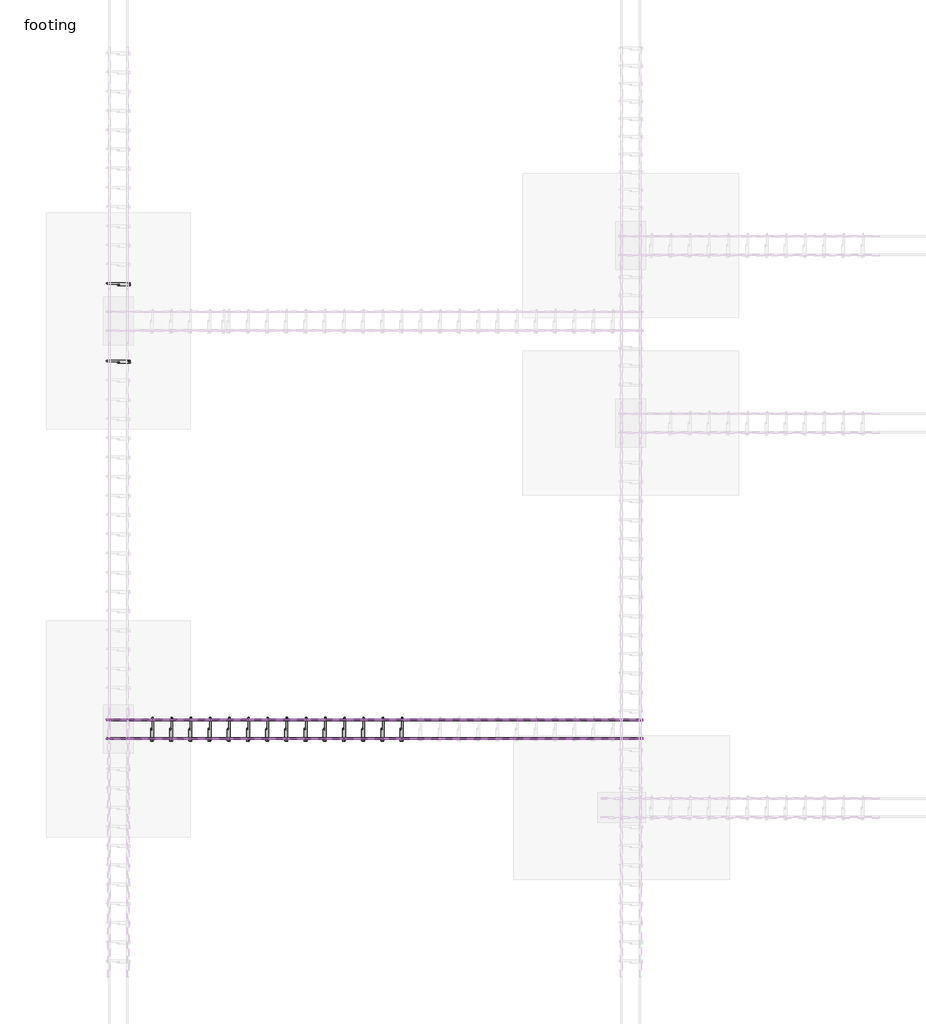
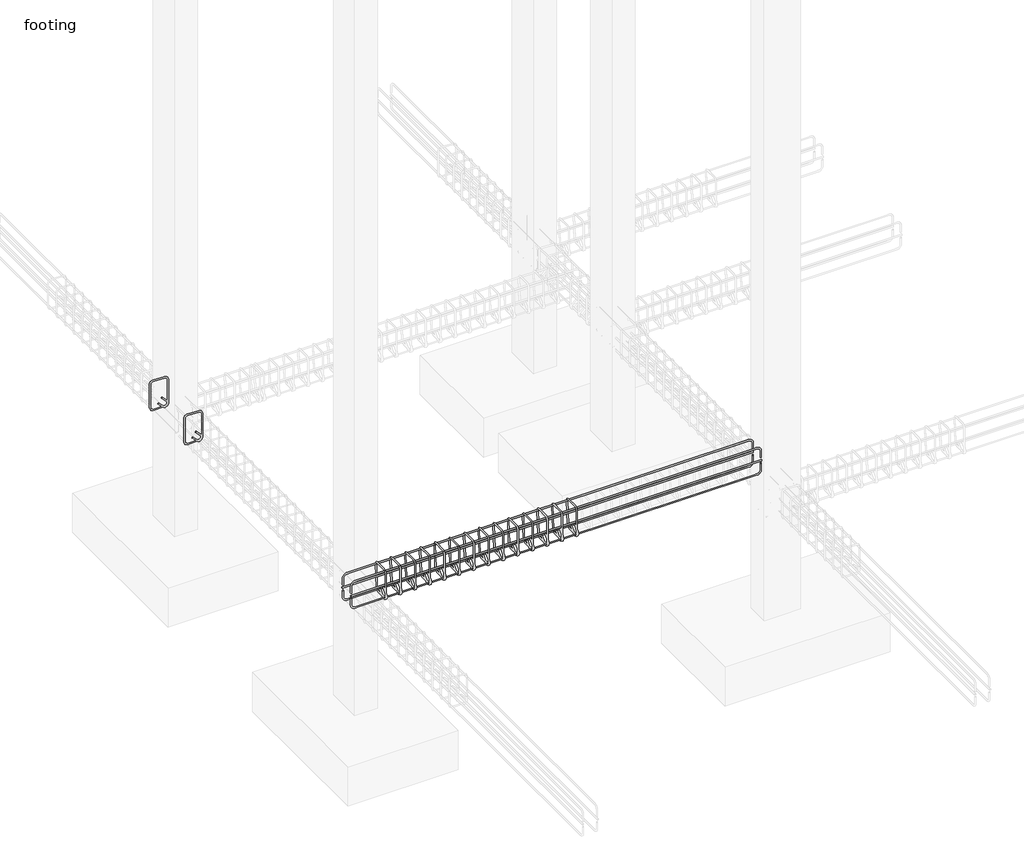
# One storey, part 6 of 21: 22 reinforcing bars.
"""IFC4 building model written with IfcOpenShell, lengths in millimetres."""

from ifc_helpers import new_model, si_unit, point, frame, origin, place, context, project, spatial, polyline, circle_curve, trimmed, segment, composite_curve, element, save
from ifc_brep_helpers import swept_disk

model = new_model("IFC4")

# Units and contexts
model_context = context("Model", 3, world=origin())
ifc_project = project(units=[si_unit("LENGTHUNIT", "METRE", prefix="MILLI")], contexts=[model_context])

# Site, building, storey
site = spatial("IfcSite", under=ifc_project)
building = spatial("IfcBuilding", under=site)
storey = spatial("IfcBuildingStorey", under=building, Name="footing", Elevation=-1524.0)

# Reinforcing bars
placement = place(None, origin())
element("IfcReinforcingBar", 1, at=placement, inside=storey, context=model_context, shape_type="SolidModel", body=[
    swept_disk(composite_curve([segment(polyline([(-10142.5883428, 4117.8887132, -310.8825168), (-10142.5883428, 4063.0237147, -365.7475153)]), True, "CONTINUOUS"), segment(trimmed(circle_curve(frame((-10142.5883428, 4040.5730744, -343.296875), z_axis=(-1.0, 0.0, 0.0), x_axis=(0.0, 22.450640299999577, -22.450640299999975)), 31.75), [point((-10142.5883428, 4063.0237147, -365.7475153))], [point((-10142.5883428, 4008.8230744, -343.296875))], True, "CARTESIAN"), True, "CONTINUOUS"), segment(polyline([(-10142.5883428, 4008.8230744, -343.296875), (-10142.5883428, 4008.8230744, -63.103125)]), True, "CONTINUOUS"), segment(trimmed(circle_curve(frame((-10142.5883428, 4040.5730744, -63.103125), z_axis=(-1.0, 0.0, 0.0), x_axis=(0.0, -31.75, 0.0)), 31.75), [point((-10142.5883428, 4008.8230744, -63.103125))], [point((-10142.5883428, 4040.5730744, -31.353125))], True, "CARTESIAN"), True, "CONTINUOUS"), segment(polyline([(-10142.5883428, 4040.5730744, -31.353125), (-10142.5883428, 4168.3668244, -31.353125)]), True, "CONTINUOUS"), segment(trimmed(circle_curve(frame((-10141.4159328, 4168.3668244, -63.0814712), z_axis=(-0.9993179916193466, 0.0, -0.03692629992126919), x_axis=(-1.1724099999992177, 0.0, 31.728346200000004)), 31.75), [point((-10142.5883428, 4168.3668244, -31.353125))], [point((-10141.4159328, 4200.1168244, -63.0814712))], True, "CARTESIAN"), True, "CONTINUOUS"), segment(polyline([(-10141.4159328, 4200.1168244, -63.0814712), (-10131.0607528, 4200.1168244, -343.3185288)]), True, "CONTINUOUS"), segment(trimmed(circle_curve(frame((-10131.0607528, 4168.3668244, -343.3185288), z_axis=(-0.9993179916193466, 0.0, -0.03692629992126919), x_axis=(0.0, 31.75, 0.0)), 31.75), [point((-10131.0607528, 4200.1168244, -343.3185288))], [point((-10129.8883428, 4168.3668244, -375.046875))], True, "CARTESIAN"), True, "CONTINUOUS"), segment(polyline([(-10129.8883428, 4168.3668244, -375.046875), (-10129.8883428, 4040.5730744, -375.046875)]), True, "CONTINUOUS"), segment(trimmed(circle_curve(frame((-10129.8883428, 4040.5730744, -343.296875), z_axis=(-1.0, 0.0, 0.0), x_axis=(0.0, 0.0, -31.75)), 31.75), [point((-10129.8883428, 4040.5730744, -375.046875))], [point((-10129.8883428, 4018.1224341, -320.8462347))], True, "CARTESIAN"), True, "CONTINUOUS"), segment(polyline([(-10129.8883428, 4018.1224341, -320.8462347), (-10129.8883428, 4072.9874326, -265.9812362)]), True, "CONTINUOUS")], self_intersect=False), 6.35),
])
element("IfcReinforcingBar", 2, at=placement, inside=storey, context=model_context, shape_type="SolidModel", body=[
    swept_disk(composite_curve([segment(polyline([(-9979.8883428, 4117.8887132, -310.8825168), (-9979.8883428, 4063.0237147, -365.7475153)]), True, "CONTINUOUS"), segment(trimmed(circle_curve(frame((-9979.8883428, 4040.5730744, -343.296875), z_axis=(-1.0, 0.0, 0.0), x_axis=(0.0, 22.450640299999577, -22.450640299999975)), 31.75), [point((-9979.8883428, 4063.0237147, -365.7475153))], [point((-9979.8883428, 4008.8230744, -343.296875))], True, "CARTESIAN"), True, "CONTINUOUS"), segment(polyline([(-9979.8883428, 4008.8230744, -343.296875), (-9979.8883428, 4008.8230744, -63.103125)]), True, "CONTINUOUS"), segment(trimmed(circle_curve(frame((-9979.8883428, 4040.5730744, -63.103125), z_axis=(-1.0, 0.0, 0.0), x_axis=(0.0, -31.75, 0.0)), 31.75), [point((-9979.8883428, 4008.8230744, -63.103125))], [point((-9979.8883428, 4040.5730744, -31.353125))], True, "CARTESIAN"), True, "CONTINUOUS"), segment(polyline([(-9979.8883428, 4040.5730744, -31.353125), (-9979.8883428, 4168.3668244, -31.353125)]), True, "CONTINUOUS"), segment(trimmed(circle_curve(frame((-9978.7159328, 4168.3668244, -63.0814712), z_axis=(-0.9993179916193466, 0.0, -0.03692629992126919), x_axis=(-1.1724100000010367, 0.0, 31.728346200000004)), 31.75), [point((-9979.8883428, 4168.3668244, -31.353125))], [point((-9978.7159328, 4200.1168244, -63.0814712))], True, "CARTESIAN"), True, "CONTINUOUS"), segment(polyline([(-9978.7159328, 4200.1168244, -63.0814712), (-9968.3607528, 4200.1168244, -343.3185288)]), True, "CONTINUOUS"), segment(trimmed(circle_curve(frame((-9968.3607528, 4168.3668244, -343.3185288), z_axis=(-0.9993179916193466, 0.0, -0.03692629992126919), x_axis=(0.0, 31.75, 0.0)), 31.75), [point((-9968.3607528, 4200.1168244, -343.3185288))], [point((-9967.1883428, 4168.3668244, -375.046875))], True, "CARTESIAN"), True, "CONTINUOUS"), segment(polyline([(-9967.1883428, 4168.3668244, -375.046875), (-9967.1883428, 4040.5730744, -375.046875)]), True, "CONTINUOUS"), segment(trimmed(circle_curve(frame((-9967.1883428, 4040.5730744, -343.296875), z_axis=(-1.0, 0.0, 0.0), x_axis=(0.0, 0.0, -31.75)), 31.75), [point((-9967.1883428, 4040.5730744, -375.046875))], [point((-9967.1883428, 4018.1224341, -320.8462347))], True, "CARTESIAN"), True, "CONTINUOUS"), segment(polyline([(-9967.1883428, 4018.1224341, -320.8462347), (-9967.1883428, 4072.9874326, -265.9812362)]), True, "CONTINUOUS")], self_intersect=False), 6.35),
])
element("IfcReinforcingBar", 3, at=placement, inside=storey, context=model_context, shape_type="SolidModel", body=[
    swept_disk(composite_curve([segment(polyline([(-9817.1883428, 4117.8887132, -310.8825168), (-9817.1883428, 4063.0237147, -365.7475153)]), True, "CONTINUOUS"), segment(trimmed(circle_curve(frame((-9817.1883428, 4040.5730744, -343.296875), z_axis=(-1.0, 0.0, 0.0), x_axis=(0.0, 22.450640299999577, -22.450640299999975)), 31.75), [point((-9817.1883428, 4063.0237147, -365.7475153))], [point((-9817.1883428, 4008.8230744, -343.296875))], True, "CARTESIAN"), True, "CONTINUOUS"), segment(polyline([(-9817.1883428, 4008.8230744, -343.296875), (-9817.1883428, 4008.8230744, -63.103125)]), True, "CONTINUOUS"), segment(trimmed(circle_curve(frame((-9817.1883428, 4040.5730744, -63.103125), z_axis=(-1.0, 0.0, 0.0), x_axis=(0.0, -31.75, 0.0)), 31.75), [point((-9817.1883428, 4008.8230744, -63.103125))], [point((-9817.1883428, 4040.5730744, -31.353125))], True, "CARTESIAN"), True, "CONTINUOUS"), segment(polyline([(-9817.1883428, 4040.5730744, -31.353125), (-9817.1883428, 4168.3668244, -31.353125)]), True, "CONTINUOUS"), segment(trimmed(circle_curve(frame((-9816.0159328, 4168.3668244, -63.0814712), z_axis=(-0.9993179916193466, 0.0, -0.03692629992126919), x_axis=(-1.1724099999992177, 0.0, 31.728346200000004)), 31.75), [point((-9817.1883428, 4168.3668244, -31.353125))], [point((-9816.0159328, 4200.1168244, -63.0814712))], True, "CARTESIAN"), True, "CONTINUOUS"), segment(polyline([(-9816.0159328, 4200.1168244, -63.0814712), (-9805.6607528, 4200.1168244, -343.3185288)]), True, "CONTINUOUS"), segment(trimmed(circle_curve(frame((-9805.6607528, 4168.3668244, -343.3185288), z_axis=(-0.9993179916193466, 0.0, -0.03692629992126919), x_axis=(0.0, 31.75, 0.0)), 31.75), [point((-9805.6607528, 4200.1168244, -343.3185288))], [point((-9804.4883428, 4168.3668244, -375.046875))], True, "CARTESIAN"), True, "CONTINUOUS"), segment(polyline([(-9804.4883428, 4168.3668244, -375.046875), (-9804.4883428, 4040.5730744, -375.046875)]), True, "CONTINUOUS"), segment(trimmed(circle_curve(frame((-9804.4883428, 4040.5730744, -343.296875), z_axis=(-1.0, 0.0, 0.0), x_axis=(0.0, 0.0, -31.75)), 31.75), [point((-9804.4883428, 4040.5730744, -375.046875))], [point((-9804.4883428, 4018.1224341, -320.8462347))], True, "CARTESIAN"), True, "CONTINUOUS"), segment(polyline([(-9804.4883428, 4018.1224341, -320.8462347), (-9804.4883428, 4072.9874326, -265.9812362)]), True, "CONTINUOUS")], self_intersect=False), 6.35),
])
element("IfcReinforcingBar", 4, at=placement, inside=storey, context=model_context, shape_type="SolidModel", body=[
    swept_disk(composite_curve([segment(polyline([(-7770.5521673, 4181.8372086, -236.1172592), (-7770.5521673, 4181.8372086, -312.3172592)]), True, "CONTINUOUS"), segment(trimmed(circle_curve(frame((-7815.0021673, 4181.8372086, -312.3172592), z_axis=(0.0, 1.0, -2.1166279873208456e-12), x_axis=(44.44999999999982, 0.0, 0.0)), 44.45), [point((-7770.5521673, 4181.8372086, -312.3172592))], [point((-7815.0021673, 4181.8372086, -356.7672592))], True, "CARTESIAN"), True, "CONTINUOUS"), segment(polyline([(-7815.0021673, 4181.8372086, -356.7672592), (-12260.7959173, 4181.8372086, -356.7672592)]), True, "CONTINUOUS"), segment(trimmed(circle_curve(frame((-12260.7959173, 4181.8372086, -312.3172592), z_axis=(0.0, 1.0, -2.1166279873208456e-12), x_axis=(0.0, 0.0, -44.44999999999999)), 44.45), [point((-12260.7959173, 4181.8372086, -356.7672592))], [point((-12305.2459173, 4181.8372086, -312.3172592))], True, "CARTESIAN"), True, "CONTINUOUS"), segment(polyline([(-12305.2459173, 4181.8372086, -312.3172592), (-12305.2459173, 4181.8372086, -236.1172592)]), True, "CONTINUOUS")], self_intersect=False), 6.35),
])
element("IfcReinforcingBar", 5, at=placement, inside=storey, context=model_context, shape_type="SolidModel", body=[
    swept_disk(composite_curve([segment(polyline([(-7770.5521673, 4027.1026902, -170.2827408), (-7770.5521673, 4027.1026902, -94.0827408)]), True, "CONTINUOUS"), segment(trimmed(circle_curve(frame((-7815.0021673, 4027.1026902, -94.0827408), z_axis=(0.0, -1.0, 0.0), x_axis=(44.44999999999982, 0.0, 0.0)), 44.45), [point((-7770.5521673, 4027.1026902, -94.0827408))], [point((-7815.0021673, 4027.1026902, -49.6327408))], True, "CARTESIAN"), True, "CONTINUOUS"), segment(polyline([(-7815.0021673, 4027.1026902, -49.6327408), (-12260.7959173, 4027.1026902, -49.6327408)]), True, "CONTINUOUS"), segment(trimmed(circle_curve(frame((-12260.7959173, 4027.1026902, -94.0827408), z_axis=(0.0, -1.0, 0.0), x_axis=(0.0, 0.0, 44.449999999999996)), 44.45), [point((-12260.7959173, 4027.1026902, -49.6327408))], [point((-12305.2459173, 4027.1026902, -94.0827408))], True, "CARTESIAN"), True, "CONTINUOUS"), segment(polyline([(-12305.2459173, 4027.1026902, -94.0827408), (-12305.2459173, 4027.1026902, -170.2827408)]), True, "CONTINUOUS")], self_intersect=False), 6.35),
])
element("IfcReinforcingBar", 6, at=placement, inside=storey, context=model_context, shape_type="SolidModel", body=[
    swept_disk(composite_curve([segment(polyline([(-7770.5521673, 4027.1026902, -236.1172592), (-7770.5521673, 4027.1026902, -312.3172592)]), True, "CONTINUOUS"), segment(trimmed(circle_curve(frame((-7815.0021673, 4027.1026902, -312.3172592), z_axis=(0.0, 1.0, 2.1166279873208456e-12), x_axis=(44.44999999999982, 0.0, 0.0)), 44.45), [point((-7770.5521673, 4027.1026902, -312.3172592))], [point((-7815.0021673, 4027.1026902, -356.7672592))], True, "CARTESIAN"), True, "CONTINUOUS"), segment(polyline([(-7815.0021673, 4027.1026902, -356.7672592), (-12260.7959173, 4027.1026902, -356.7672592)]), True, "CONTINUOUS"), segment(trimmed(circle_curve(frame((-12260.7959173, 4027.1026902, -312.3172592), z_axis=(0.0, 1.0, 2.1166279873208456e-12), x_axis=(0.0, 0.0, -44.44999999999999)), 44.45), [point((-12260.7959173, 4027.1026902, -356.7672592))], [point((-12305.2459173, 4027.1026902, -312.3172592))], True, "CARTESIAN"), True, "CONTINUOUS"), segment(polyline([(-12305.2459173, 4027.1026902, -312.3172592), (-12305.2459173, 4027.1026902, -236.1172592)]), True, "CONTINUOUS")], self_intersect=False), 6.35),
])
element("IfcReinforcingBar", 7, at=placement, inside=storey, context=model_context, shape_type="SolidModel", body=[
    swept_disk(composite_curve([segment(polyline([(-7770.5521673, 4181.8372086, -170.2827408), (-7770.5521673, 4181.8372086, -94.0827408)]), True, "CONTINUOUS"), segment(trimmed(circle_curve(frame((-7815.0021673, 4181.8372086, -94.0827408), z_axis=(0.0, -1.0, 0.0), x_axis=(44.44999999999982, 0.0, 0.0)), 44.45), [point((-7770.5521673, 4181.8372086, -94.0827408))], [point((-7815.0021673, 4181.8372086, -49.6327408))], True, "CARTESIAN"), True, "CONTINUOUS"), segment(polyline([(-7815.0021673, 4181.8372086, -49.6327408), (-12260.7959173, 4181.8372086, -49.6327408)]), True, "CONTINUOUS"), segment(trimmed(circle_curve(frame((-12260.7959173, 4181.8372086, -94.0827408), z_axis=(0.0, -1.0, 0.0), x_axis=(0.0, 0.0, 44.449999999999996)), 44.45), [point((-12260.7959173, 4181.8372086, -49.6327408))], [point((-12305.2459173, 4181.8372086, -94.0827408))], True, "CARTESIAN"), True, "CONTINUOUS"), segment(polyline([(-12305.2459173, 4181.8372086, -94.0827408), (-12305.2459173, 4181.8372086, -170.2827408)]), True, "CONTINUOUS")], self_intersect=False), 6.35),
])
element("IfcReinforcingBar", 8, at=placement, inside=storey, context=model_context, shape_type="SolidModel", body=[
    swept_disk(composite_curve([segment(polyline([(-7764.2021673, 4187.4168244, -203.2), (-12311.5959173, 4187.4168244, -203.2)]), True, "CONTINUOUS")], self_intersect=False), 6.35),
])
element("IfcReinforcingBar", 9, at=placement, inside=storey, context=model_context, shape_type="SolidModel", body=[
    swept_disk(composite_curve([segment(polyline([(-7764.2021673, 4021.5230744, -203.2), (-12311.5959173, 4021.5230744, -203.2)]), True, "CONTINUOUS")], self_intersect=False), 6.35),
])
element("IfcReinforcingBar", 10, at=placement, inside=storey, context=model_context, shape_type="SolidModel", body=[
    swept_disk(composite_curve([segment(polyline([(-10305.2883428, 4117.8887132, -310.8825168), (-10305.2883428, 4063.0237147, -365.7475153)]), True, "CONTINUOUS"), segment(trimmed(circle_curve(frame((-10305.2883428, 4040.5730744, -343.296875), z_axis=(-1.0, 0.0, 0.0), x_axis=(0.0, 22.450640299999577, -22.450640299999975)), 31.75), [point((-10305.2883428, 4063.0237147, -365.7475153))], [point((-10305.2883428, 4008.8230744, -343.296875))], True, "CARTESIAN"), True, "CONTINUOUS"), segment(polyline([(-10305.2883428, 4008.8230744, -343.296875), (-10305.2883428, 4008.8230744, -63.103125)]), True, "CONTINUOUS"), segment(trimmed(circle_curve(frame((-10305.2883428, 4040.5730744, -63.103125), z_axis=(-1.0, 0.0, 0.0), x_axis=(0.0, -31.75, 0.0)), 31.75), [point((-10305.2883428, 4008.8230744, -63.103125))], [point((-10305.2883428, 4040.5730744, -31.353125))], True, "CARTESIAN"), True, "CONTINUOUS"), segment(polyline([(-10305.2883428, 4040.5730744, -31.353125), (-10305.2883428, 4168.3668244, -31.353125)]), True, "CONTINUOUS"), segment(trimmed(circle_curve(frame((-10304.1159328, 4168.3668244, -63.0814712), z_axis=(-0.9993179916193466, 0.0, -0.03692629992126919), x_axis=(-1.1724100000010367, 0.0, 31.728346200000004)), 31.75), [point((-10305.2883428, 4168.3668244, -31.353125))], [point((-10304.1159328, 4200.1168244, -63.0814712))], True, "CARTESIAN"), True, "CONTINUOUS"), segment(polyline([(-10304.1159328, 4200.1168244, -63.0814712), (-10293.7607528, 4200.1168244, -343.3185288)]), True, "CONTINUOUS"), segment(trimmed(circle_curve(frame((-10293.7607528, 4168.3668244, -343.3185288), z_axis=(-0.9993179916193466, 0.0, -0.03692629992126919), x_axis=(0.0, 31.75, 0.0)), 31.75), [point((-10293.7607528, 4200.1168244, -343.3185288))], [point((-10292.5883428, 4168.3668244, -375.046875))], True, "CARTESIAN"), True, "CONTINUOUS"), segment(polyline([(-10292.5883428, 4168.3668244, -375.046875), (-10292.5883428, 4040.5730744, -375.046875)]), True, "CONTINUOUS"), segment(trimmed(circle_curve(frame((-10292.5883428, 4040.5730744, -343.296875), z_axis=(-1.0, 0.0, 0.0), x_axis=(0.0, 0.0, -31.75)), 31.75), [point((-10292.5883428, 4040.5730744, -375.046875))], [point((-10292.5883428, 4018.1224341, -320.8462347))], True, "CARTESIAN"), True, "CONTINUOUS"), segment(polyline([(-10292.5883428, 4018.1224341, -320.8462347), (-10292.5883428, 4072.9874326, -265.9812362)]), True, "CONTINUOUS")], self_intersect=False), 6.35),
])
element("IfcReinforcingBar", 11, at=placement, inside=storey, context=model_context, shape_type="SolidModel", body=[
    swept_disk(composite_curve([segment(polyline([(-10467.9883428, 4117.8887132, -310.8825168), (-10467.9883428, 4063.0237147, -365.7475153)]), True, "CONTINUOUS"), segment(trimmed(circle_curve(frame((-10467.9883428, 4040.5730744, -343.296875), z_axis=(-1.0, 0.0, 0.0), x_axis=(0.0, 22.450640299999577, -22.450640299999975)), 31.75), [point((-10467.9883428, 4063.0237147, -365.7475153))], [point((-10467.9883428, 4008.8230744, -343.296875))], True, "CARTESIAN"), True, "CONTINUOUS"), segment(polyline([(-10467.9883428, 4008.8230744, -343.296875), (-10467.9883428, 4008.8230744, -63.103125)]), True, "CONTINUOUS"), segment(trimmed(circle_curve(frame((-10467.9883428, 4040.5730744, -63.103125), z_axis=(-1.0, 0.0, 0.0), x_axis=(0.0, -31.75, 0.0)), 31.75), [point((-10467.9883428, 4008.8230744, -63.103125))], [point((-10467.9883428, 4040.5730744, -31.353125))], True, "CARTESIAN"), True, "CONTINUOUS"), segment(polyline([(-10467.9883428, 4040.5730744, -31.353125), (-10467.9883428, 4168.3668244, -31.353125)]), True, "CONTINUOUS"), segment(trimmed(circle_curve(frame((-10466.8159328, 4168.3668244, -63.0814712), z_axis=(-0.9993179916193466, 0.0, -0.03692629992126919), x_axis=(-1.1724099999992177, 0.0, 31.728346200000004)), 31.75), [point((-10467.9883428, 4168.3668244, -31.353125))], [point((-10466.8159328, 4200.1168244, -63.0814712))], True, "CARTESIAN"), True, "CONTINUOUS"), segment(polyline([(-10466.8159328, 4200.1168244, -63.0814712), (-10456.4607528, 4200.1168244, -343.3185288)]), True, "CONTINUOUS"), segment(trimmed(circle_curve(frame((-10456.4607528, 4168.3668244, -343.3185288), z_axis=(-0.9993179916193466, 0.0, -0.03692629992126919), x_axis=(0.0, 31.75, 0.0)), 31.75), [point((-10456.4607528, 4200.1168244, -343.3185288))], [point((-10455.2883428, 4168.3668244, -375.046875))], True, "CARTESIAN"), True, "CONTINUOUS"), segment(polyline([(-10455.2883428, 4168.3668244, -375.046875), (-10455.2883428, 4040.5730744, -375.046875)]), True, "CONTINUOUS"), segment(trimmed(circle_curve(frame((-10455.2883428, 4040.5730744, -343.296875), z_axis=(-1.0, 0.0, 0.0), x_axis=(0.0, 0.0, -31.75)), 31.75), [point((-10455.2883428, 4040.5730744, -375.046875))], [point((-10455.2883428, 4018.1224341, -320.8462347))], True, "CARTESIAN"), True, "CONTINUOUS"), segment(polyline([(-10455.2883428, 4018.1224341, -320.8462347), (-10455.2883428, 4072.9874326, -265.9812362)]), True, "CONTINUOUS")], self_intersect=False), 6.35),
])
element("IfcReinforcingBar", 12, at=placement, inside=storey, context=model_context, shape_type="SolidModel", body=[
    swept_disk(composite_curve([segment(polyline([(-10630.6883428, 4117.8887132, -310.8825168), (-10630.6883428, 4063.0237147, -365.7475153)]), True, "CONTINUOUS"), segment(trimmed(circle_curve(frame((-10630.6883428, 4040.5730744, -343.296875), z_axis=(-1.0, 0.0, 0.0), x_axis=(0.0, 22.450640299999577, -22.450640299999975)), 31.75), [point((-10630.6883428, 4063.0237147, -365.7475153))], [point((-10630.6883428, 4008.8230744, -343.296875))], True, "CARTESIAN"), True, "CONTINUOUS"), segment(polyline([(-10630.6883428, 4008.8230744, -343.296875), (-10630.6883428, 4008.8230744, -63.103125)]), True, "CONTINUOUS"), segment(trimmed(circle_curve(frame((-10630.6883428, 4040.5730744, -63.103125), z_axis=(-1.0, 0.0, 0.0), x_axis=(0.0, -31.75, 0.0)), 31.75), [point((-10630.6883428, 4008.8230744, -63.103125))], [point((-10630.6883428, 4040.5730744, -31.353125))], True, "CARTESIAN"), True, "CONTINUOUS"), segment(polyline([(-10630.6883428, 4040.5730744, -31.353125), (-10630.6883428, 4168.3668244, -31.353125)]), True, "CONTINUOUS"), segment(trimmed(circle_curve(frame((-10629.5159328, 4168.3668244, -63.0814712), z_axis=(-0.9993179916193466, 0.0, -0.03692629992126919), x_axis=(-1.1724099999992177, 0.0, 31.728346200000004)), 31.75), [point((-10630.6883428, 4168.3668244, -31.353125))], [point((-10629.5159328, 4200.1168244, -63.0814712))], True, "CARTESIAN"), True, "CONTINUOUS"), segment(polyline([(-10629.5159328, 4200.1168244, -63.0814712), (-10619.1607528, 4200.1168244, -343.3185288)]), True, "CONTINUOUS"), segment(trimmed(circle_curve(frame((-10619.1607528, 4168.3668244, -343.3185288), z_axis=(-0.9993179916193466, 0.0, -0.03692629992126919), x_axis=(0.0, 31.75, 0.0)), 31.75), [point((-10619.1607528, 4200.1168244, -343.3185288))], [point((-10617.9883428, 4168.3668244, -375.046875))], True, "CARTESIAN"), True, "CONTINUOUS"), segment(polyline([(-10617.9883428, 4168.3668244, -375.046875), (-10617.9883428, 4040.5730744, -375.046875)]), True, "CONTINUOUS"), segment(trimmed(circle_curve(frame((-10617.9883428, 4040.5730744, -343.296875), z_axis=(-1.0, 0.0, 0.0), x_axis=(0.0, 0.0, -31.75)), 31.75), [point((-10617.9883428, 4040.5730744, -375.046875))], [point((-10617.9883428, 4018.1224341, -320.8462347))], True, "CARTESIAN"), True, "CONTINUOUS"), segment(polyline([(-10617.9883428, 4018.1224341, -320.8462347), (-10617.9883428, 4072.9874326, -265.9812362)]), True, "CONTINUOUS")], self_intersect=False), 6.35),
])
element("IfcReinforcingBar", 13, at=placement, inside=storey, context=model_context, shape_type="SolidModel", body=[
    swept_disk(composite_curve([segment(polyline([(-10793.3883428, 4117.8887132, -310.8825168), (-10793.3883428, 4063.0237147, -365.7475153)]), True, "CONTINUOUS"), segment(trimmed(circle_curve(frame((-10793.3883428, 4040.5730744, -343.296875), z_axis=(-1.0, 0.0, 0.0), x_axis=(0.0, 22.450640299999577, -22.450640299999975)), 31.75), [point((-10793.3883428, 4063.0237147, -365.7475153))], [point((-10793.3883428, 4008.8230744, -343.296875))], True, "CARTESIAN"), True, "CONTINUOUS"), segment(polyline([(-10793.3883428, 4008.8230744, -343.296875), (-10793.3883428, 4008.8230744, -63.103125)]), True, "CONTINUOUS"), segment(trimmed(circle_curve(frame((-10793.3883428, 4040.5730744, -63.103125), z_axis=(-1.0, 0.0, 0.0), x_axis=(0.0, -31.75, 0.0)), 31.75), [point((-10793.3883428, 4008.8230744, -63.103125))], [point((-10793.3883428, 4040.5730744, -31.353125))], True, "CARTESIAN"), True, "CONTINUOUS"), segment(polyline([(-10793.3883428, 4040.5730744, -31.353125), (-10793.3883428, 4168.3668244, -31.353125)]), True, "CONTINUOUS"), segment(trimmed(circle_curve(frame((-10792.2159328, 4168.3668244, -63.0814712), z_axis=(-0.9993179916193466, 0.0, -0.03692629992126919), x_axis=(-1.1724100000010367, 0.0, 31.728346200000004)), 31.75), [point((-10793.3883428, 4168.3668244, -31.353125))], [point((-10792.2159328, 4200.1168244, -63.0814712))], True, "CARTESIAN"), True, "CONTINUOUS"), segment(polyline([(-10792.2159328, 4200.1168244, -63.0814712), (-10781.8607528, 4200.1168244, -343.3185288)]), True, "CONTINUOUS"), segment(trimmed(circle_curve(frame((-10781.8607528, 4168.3668244, -343.3185288), z_axis=(-0.9993179916193466, 0.0, -0.03692629992126919), x_axis=(0.0, 31.75, 0.0)), 31.75), [point((-10781.8607528, 4200.1168244, -343.3185288))], [point((-10780.6883428, 4168.3668244, -375.046875))], True, "CARTESIAN"), True, "CONTINUOUS"), segment(polyline([(-10780.6883428, 4168.3668244, -375.046875), (-10780.6883428, 4040.5730744, -375.046875)]), True, "CONTINUOUS"), segment(trimmed(circle_curve(frame((-10780.6883428, 4040.5730744, -343.296875), z_axis=(-1.0, 0.0, 0.0), x_axis=(0.0, 0.0, -31.75)), 31.75), [point((-10780.6883428, 4040.5730744, -375.046875))], [point((-10780.6883428, 4018.1224341, -320.8462347))], True, "CARTESIAN"), True, "CONTINUOUS"), segment(polyline([(-10780.6883428, 4018.1224341, -320.8462347), (-10780.6883428, 4072.9874326, -265.9812362)]), True, "CONTINUOUS")], self_intersect=False), 6.35),
])
element("IfcReinforcingBar", 14, at=placement, inside=storey, context=model_context, shape_type="SolidModel", body=[
    swept_disk(composite_curve([segment(polyline([(-10956.0883428, 4117.8887132, -310.8825168), (-10956.0883428, 4063.0237147, -365.7475153)]), True, "CONTINUOUS"), segment(trimmed(circle_curve(frame((-10956.0883428, 4040.5730744, -343.296875), z_axis=(-1.0, 0.0, 0.0), x_axis=(0.0, 22.450640299999577, -22.450640299999975)), 31.75), [point((-10956.0883428, 4063.0237147, -365.7475153))], [point((-10956.0883428, 4008.8230744, -343.296875))], True, "CARTESIAN"), True, "CONTINUOUS"), segment(polyline([(-10956.0883428, 4008.8230744, -343.296875), (-10956.0883428, 4008.8230744, -63.103125)]), True, "CONTINUOUS"), segment(trimmed(circle_curve(frame((-10956.0883428, 4040.5730744, -63.103125), z_axis=(-1.0, 0.0, 0.0), x_axis=(0.0, -31.75, 0.0)), 31.75), [point((-10956.0883428, 4008.8230744, -63.103125))], [point((-10956.0883428, 4040.5730744, -31.353125))], True, "CARTESIAN"), True, "CONTINUOUS"), segment(polyline([(-10956.0883428, 4040.5730744, -31.353125), (-10956.0883428, 4168.3668244, -31.353125)]), True, "CONTINUOUS"), segment(trimmed(circle_curve(frame((-10954.9159328, 4168.3668244, -63.0814712), z_axis=(-0.9993179916193466, 0.0, -0.03692629992126919), x_axis=(-1.1724099999992177, 0.0, 31.728346200000004)), 31.75), [point((-10956.0883428, 4168.3668244, -31.353125))], [point((-10954.9159328, 4200.1168244, -63.0814712))], True, "CARTESIAN"), True, "CONTINUOUS"), segment(polyline([(-10954.9159328, 4200.1168244, -63.0814712), (-10944.5607528, 4200.1168244, -343.3185288)]), True, "CONTINUOUS"), segment(trimmed(circle_curve(frame((-10944.5607528, 4168.3668244, -343.3185288), z_axis=(-0.9993179916193466, 0.0, -0.03692629992126919), x_axis=(0.0, 31.75, 0.0)), 31.75), [point((-10944.5607528, 4200.1168244, -343.3185288))], [point((-10943.3883428, 4168.3668244, -375.046875))], True, "CARTESIAN"), True, "CONTINUOUS"), segment(polyline([(-10943.3883428, 4168.3668244, -375.046875), (-10943.3883428, 4040.5730744, -375.046875)]), True, "CONTINUOUS"), segment(trimmed(circle_curve(frame((-10943.3883428, 4040.5730744, -343.296875), z_axis=(-1.0, 0.0, 0.0), x_axis=(0.0, 0.0, -31.75)), 31.75), [point((-10943.3883428, 4040.5730744, -375.046875))], [point((-10943.3883428, 4018.1224341, -320.8462347))], True, "CARTESIAN"), True, "CONTINUOUS"), segment(polyline([(-10943.3883428, 4018.1224341, -320.8462347), (-10943.3883428, 4072.9874326, -265.9812362)]), True, "CONTINUOUS")], self_intersect=False), 6.35),
])
element("IfcReinforcingBar", 15, at=placement, inside=storey, context=model_context, shape_type="SolidModel", body=[
    swept_disk(composite_curve([segment(polyline([(-11118.7883428, 4117.8887132, -310.8825168), (-11118.7883428, 4063.0237147, -365.7475153)]), True, "CONTINUOUS"), segment(trimmed(circle_curve(frame((-11118.7883428, 4040.5730744, -343.296875), z_axis=(-1.0, 0.0, 0.0), x_axis=(0.0, 22.450640299999577, -22.450640299999975)), 31.75), [point((-11118.7883428, 4063.0237147, -365.7475153))], [point((-11118.7883428, 4008.8230744, -343.296875))], True, "CARTESIAN"), True, "CONTINUOUS"), segment(polyline([(-11118.7883428, 4008.8230744, -343.296875), (-11118.7883428, 4008.8230744, -63.103125)]), True, "CONTINUOUS"), segment(trimmed(circle_curve(frame((-11118.7883428, 4040.5730744, -63.103125), z_axis=(-1.0, 0.0, 0.0), x_axis=(0.0, -31.75, 0.0)), 31.75), [point((-11118.7883428, 4008.8230744, -63.103125))], [point((-11118.7883428, 4040.5730744, -31.353125))], True, "CARTESIAN"), True, "CONTINUOUS"), segment(polyline([(-11118.7883428, 4040.5730744, -31.353125), (-11118.7883428, 4168.3668244, -31.353125)]), True, "CONTINUOUS"), segment(trimmed(circle_curve(frame((-11117.6159328, 4168.3668244, -63.0814712), z_axis=(-0.9993179916193466, 0.0, -0.03692629992126919), x_axis=(-1.1724100000010367, 0.0, 31.728346200000004)), 31.75), [point((-11118.7883428, 4168.3668244, -31.353125))], [point((-11117.6159328, 4200.1168244, -63.0814712))], True, "CARTESIAN"), True, "CONTINUOUS"), segment(polyline([(-11117.6159328, 4200.1168244, -63.0814712), (-11107.2607528, 4200.1168244, -343.3185288)]), True, "CONTINUOUS"), segment(trimmed(circle_curve(frame((-11107.2607528, 4168.3668244, -343.3185288), z_axis=(-0.9993179916193466, 0.0, -0.03692629992126919), x_axis=(0.0, 31.75, 0.0)), 31.75), [point((-11107.2607528, 4200.1168244, -343.3185288))], [point((-11106.0883428, 4168.3668244, -375.046875))], True, "CARTESIAN"), True, "CONTINUOUS"), segment(polyline([(-11106.0883428, 4168.3668244, -375.046875), (-11106.0883428, 4040.5730744, -375.046875)]), True, "CONTINUOUS"), segment(trimmed(circle_curve(frame((-11106.0883428, 4040.5730744, -343.296875), z_axis=(-1.0, 0.0, 0.0), x_axis=(0.0, 0.0, -31.75)), 31.75), [point((-11106.0883428, 4040.5730744, -375.046875))], [point((-11106.0883428, 4018.1224341, -320.8462347))], True, "CARTESIAN"), True, "CONTINUOUS"), segment(polyline([(-11106.0883428, 4018.1224341, -320.8462347), (-11106.0883428, 4072.9874326, -265.9812362)]), True, "CONTINUOUS")], self_intersect=False), 6.35),
])
element("IfcReinforcingBar", 16, at=placement, inside=storey, context=model_context, shape_type="SolidModel", body=[
    swept_disk(composite_curve([segment(polyline([(-11281.4883428, 4117.8887132, -310.8825168), (-11281.4883428, 4063.0237147, -365.7475153)]), True, "CONTINUOUS"), segment(trimmed(circle_curve(frame((-11281.4883428, 4040.5730744, -343.296875), z_axis=(-1.0, 0.0, 0.0), x_axis=(0.0, 22.450640299999577, -22.450640299999975)), 31.75), [point((-11281.4883428, 4063.0237147, -365.7475153))], [point((-11281.4883428, 4008.8230744, -343.296875))], True, "CARTESIAN"), True, "CONTINUOUS"), segment(polyline([(-11281.4883428, 4008.8230744, -343.296875), (-11281.4883428, 4008.8230744, -63.103125)]), True, "CONTINUOUS"), segment(trimmed(circle_curve(frame((-11281.4883428, 4040.5730744, -63.103125), z_axis=(-1.0, 0.0, 0.0), x_axis=(0.0, -31.75, 0.0)), 31.75), [point((-11281.4883428, 4008.8230744, -63.103125))], [point((-11281.4883428, 4040.5730744, -31.353125))], True, "CARTESIAN"), True, "CONTINUOUS"), segment(polyline([(-11281.4883428, 4040.5730744, -31.353125), (-11281.4883428, 4168.3668244, -31.353125)]), True, "CONTINUOUS"), segment(trimmed(circle_curve(frame((-11280.3159328, 4168.3668244, -63.0814712), z_axis=(-0.9993179916193466, 0.0, -0.03692629992126919), x_axis=(-1.1724099999992177, 0.0, 31.728346200000004)), 31.75), [point((-11281.4883428, 4168.3668244, -31.353125))], [point((-11280.3159328, 4200.1168244, -63.0814712))], True, "CARTESIAN"), True, "CONTINUOUS"), segment(polyline([(-11280.3159328, 4200.1168244, -63.0814712), (-11269.9607528, 4200.1168244, -343.3185288)]), True, "CONTINUOUS"), segment(trimmed(circle_curve(frame((-11269.9607528, 4168.3668244, -343.3185288), z_axis=(-0.9993179916193466, 0.0, -0.03692629992126919), x_axis=(0.0, 31.75, 0.0)), 31.75), [point((-11269.9607528, 4200.1168244, -343.3185288))], [point((-11268.7883428, 4168.3668244, -375.046875))], True, "CARTESIAN"), True, "CONTINUOUS"), segment(polyline([(-11268.7883428, 4168.3668244, -375.046875), (-11268.7883428, 4040.5730744, -375.046875)]), True, "CONTINUOUS"), segment(trimmed(circle_curve(frame((-11268.7883428, 4040.5730744, -343.296875), z_axis=(-1.0, 0.0, 0.0), x_axis=(0.0, 0.0, -31.75)), 31.75), [point((-11268.7883428, 4040.5730744, -375.046875))], [point((-11268.7883428, 4018.1224341, -320.8462347))], True, "CARTESIAN"), True, "CONTINUOUS"), segment(polyline([(-11268.7883428, 4018.1224341, -320.8462347), (-11268.7883428, 4072.9874326, -265.9812362)]), True, "CONTINUOUS")], self_intersect=False), 6.35),
])
element("IfcReinforcingBar", 17, at=placement, inside=storey, context=model_context, shape_type="SolidModel", body=[
    swept_disk(composite_curve([segment(polyline([(-11444.1883428, 4117.8887132, -310.8825168), (-11444.1883428, 4063.0237147, -365.7475153)]), True, "CONTINUOUS"), segment(trimmed(circle_curve(frame((-11444.1883428, 4040.5730744, -343.296875), z_axis=(-1.0, 0.0, 0.0), x_axis=(0.0, 22.450640299999577, -22.450640299999975)), 31.75), [point((-11444.1883428, 4063.0237147, -365.7475153))], [point((-11444.1883428, 4008.8230744, -343.296875))], True, "CARTESIAN"), True, "CONTINUOUS"), segment(polyline([(-11444.1883428, 4008.8230744, -343.296875), (-11444.1883428, 4008.8230744, -63.103125)]), True, "CONTINUOUS"), segment(trimmed(circle_curve(frame((-11444.1883428, 4040.5730744, -63.103125), z_axis=(-1.0, 0.0, 0.0), x_axis=(0.0, -31.75, 0.0)), 31.75), [point((-11444.1883428, 4008.8230744, -63.103125))], [point((-11444.1883428, 4040.5730744, -31.353125))], True, "CARTESIAN"), True, "CONTINUOUS"), segment(polyline([(-11444.1883428, 4040.5730744, -31.353125), (-11444.1883428, 4168.3668244, -31.353125)]), True, "CONTINUOUS"), segment(trimmed(circle_curve(frame((-11443.0159328, 4168.3668244, -63.0814712), z_axis=(-0.9993179916193466, 0.0, -0.03692629992126919), x_axis=(-1.1724099999992177, 0.0, 31.728346200000004)), 31.75), [point((-11444.1883428, 4168.3668244, -31.353125))], [point((-11443.0159328, 4200.1168244, -63.0814712))], True, "CARTESIAN"), True, "CONTINUOUS"), segment(polyline([(-11443.0159328, 4200.1168244, -63.0814712), (-11432.6607528, 4200.1168244, -343.3185288)]), True, "CONTINUOUS"), segment(trimmed(circle_curve(frame((-11432.6607528, 4168.3668244, -343.3185288), z_axis=(-0.9993179916193466, 0.0, -0.03692629992126919), x_axis=(0.0, 31.75, 0.0)), 31.75), [point((-11432.6607528, 4200.1168244, -343.3185288))], [point((-11431.4883428, 4168.3668244, -375.046875))], True, "CARTESIAN"), True, "CONTINUOUS"), segment(polyline([(-11431.4883428, 4168.3668244, -375.046875), (-11431.4883428, 4040.5730744, -375.046875)]), True, "CONTINUOUS"), segment(trimmed(circle_curve(frame((-11431.4883428, 4040.5730744, -343.296875), z_axis=(-1.0, 0.0, 0.0), x_axis=(0.0, 0.0, -31.75)), 31.75), [point((-11431.4883428, 4040.5730744, -375.046875))], [point((-11431.4883428, 4018.1224341, -320.8462347))], True, "CARTESIAN"), True, "CONTINUOUS"), segment(polyline([(-11431.4883428, 4018.1224341, -320.8462347), (-11431.4883428, 4072.9874326, -265.9812362)]), True, "CONTINUOUS")], self_intersect=False), 6.35),
])
element("IfcReinforcingBar", 18, at=placement, inside=storey, context=model_context, shape_type="SolidModel", body=[
    swept_disk(composite_curve([segment(polyline([(-11606.8883428, 4117.8887132, -310.8825168), (-11606.8883428, 4063.0237147, -365.7475153)]), True, "CONTINUOUS"), segment(trimmed(circle_curve(frame((-11606.8883428, 4040.5730744, -343.296875), z_axis=(-1.0, 0.0, 0.0), x_axis=(0.0, 22.450640299999577, -22.450640299999975)), 31.75), [point((-11606.8883428, 4063.0237147, -365.7475153))], [point((-11606.8883428, 4008.8230744, -343.296875))], True, "CARTESIAN"), True, "CONTINUOUS"), segment(polyline([(-11606.8883428, 4008.8230744, -343.296875), (-11606.8883428, 4008.8230744, -63.103125)]), True, "CONTINUOUS"), segment(trimmed(circle_curve(frame((-11606.8883428, 4040.5730744, -63.103125), z_axis=(-1.0, 0.0, 0.0), x_axis=(0.0, -31.75, 0.0)), 31.75), [point((-11606.8883428, 4008.8230744, -63.103125))], [point((-11606.8883428, 4040.5730744, -31.353125))], True, "CARTESIAN"), True, "CONTINUOUS"), segment(polyline([(-11606.8883428, 4040.5730744, -31.353125), (-11606.8883428, 4168.3668244, -31.353125)]), True, "CONTINUOUS"), segment(trimmed(circle_curve(frame((-11605.7159328, 4168.3668244, -63.0814712), z_axis=(-0.9993179916193466, 0.0, -0.03692629992126919), x_axis=(-1.1724100000010367, 0.0, 31.728346200000004)), 31.75), [point((-11606.8883428, 4168.3668244, -31.353125))], [point((-11605.7159328, 4200.1168244, -63.0814712))], True, "CARTESIAN"), True, "CONTINUOUS"), segment(polyline([(-11605.7159328, 4200.1168244, -63.0814712), (-11595.3607528, 4200.1168244, -343.3185288)]), True, "CONTINUOUS"), segment(trimmed(circle_curve(frame((-11595.3607528, 4168.3668244, -343.3185288), z_axis=(-0.9993179916193466, 0.0, -0.03692629992126919), x_axis=(0.0, 31.75, 0.0)), 31.75), [point((-11595.3607528, 4200.1168244, -343.3185288))], [point((-11594.1883428, 4168.3668244, -375.046875))], True, "CARTESIAN"), True, "CONTINUOUS"), segment(polyline([(-11594.1883428, 4168.3668244, -375.046875), (-11594.1883428, 4040.5730744, -375.046875)]), True, "CONTINUOUS"), segment(trimmed(circle_curve(frame((-11594.1883428, 4040.5730744, -343.296875), z_axis=(-1.0, 0.0, 0.0), x_axis=(0.0, 0.0, -31.75)), 31.75), [point((-11594.1883428, 4040.5730744, -375.046875))], [point((-11594.1883428, 4018.1224341, -320.8462347))], True, "CARTESIAN"), True, "CONTINUOUS"), segment(polyline([(-11594.1883428, 4018.1224341, -320.8462347), (-11594.1883428, 4072.9874326, -265.9812362)]), True, "CONTINUOUS")], self_intersect=False), 6.35),
])
element("IfcReinforcingBar", 19, at=placement, inside=storey, context=model_context, shape_type="SolidModel", body=[
    swept_disk(composite_curve([segment(polyline([(-11769.5883428, 4117.8887132, -310.8825168), (-11769.5883428, 4063.0237147, -365.7475153)]), True, "CONTINUOUS"), segment(trimmed(circle_curve(frame((-11769.5883428, 4040.5730744, -343.296875), z_axis=(-1.0, 0.0, 0.0), x_axis=(0.0, 22.450640299999577, -22.450640299999975)), 31.75), [point((-11769.5883428, 4063.0237147, -365.7475153))], [point((-11769.5883428, 4008.8230744, -343.296875))], True, "CARTESIAN"), True, "CONTINUOUS"), segment(polyline([(-11769.5883428, 4008.8230744, -343.296875), (-11769.5883428, 4008.8230744, -63.103125)]), True, "CONTINUOUS"), segment(trimmed(circle_curve(frame((-11769.5883428, 4040.5730744, -63.103125), z_axis=(-1.0, 0.0, 0.0), x_axis=(0.0, -31.75, 0.0)), 31.75), [point((-11769.5883428, 4008.8230744, -63.103125))], [point((-11769.5883428, 4040.5730744, -31.353125))], True, "CARTESIAN"), True, "CONTINUOUS"), segment(polyline([(-11769.5883428, 4040.5730744, -31.353125), (-11769.5883428, 4168.3668244, -31.353125)]), True, "CONTINUOUS"), segment(trimmed(circle_curve(frame((-11768.4159328, 4168.3668244, -63.0814712), z_axis=(-0.9993179916193466, 0.0, -0.03692629992126919), x_axis=(-1.1724099999992177, 0.0, 31.728346200000004)), 31.75), [point((-11769.5883428, 4168.3668244, -31.353125))], [point((-11768.4159328, 4200.1168244, -63.0814712))], True, "CARTESIAN"), True, "CONTINUOUS"), segment(polyline([(-11768.4159328, 4200.1168244, -63.0814712), (-11758.0607528, 4200.1168244, -343.3185288)]), True, "CONTINUOUS"), segment(trimmed(circle_curve(frame((-11758.0607528, 4168.3668244, -343.3185288), z_axis=(-0.9993179916193466, 0.0, -0.03692629992126919), x_axis=(0.0, 31.75, 0.0)), 31.75), [point((-11758.0607528, 4200.1168244, -343.3185288))], [point((-11756.8883428, 4168.3668244, -375.046875))], True, "CARTESIAN"), True, "CONTINUOUS"), segment(polyline([(-11756.8883428, 4168.3668244, -375.046875), (-11756.8883428, 4040.5730744, -375.046875)]), True, "CONTINUOUS"), segment(trimmed(circle_curve(frame((-11756.8883428, 4040.5730744, -343.296875), z_axis=(-1.0, 0.0, 0.0), x_axis=(0.0, 0.0, -31.75)), 31.75), [point((-11756.8883428, 4040.5730744, -375.046875))], [point((-11756.8883428, 4018.1224341, -320.8462347))], True, "CARTESIAN"), True, "CONTINUOUS"), segment(polyline([(-11756.8883428, 4018.1224341, -320.8462347), (-11756.8883428, 4072.9874326, -265.9812362)]), True, "CONTINUOUS")], self_intersect=False), 6.35),
])
element("IfcReinforcingBar", 20, at=placement, inside=storey, context=model_context, shape_type="SolidModel", body=[
    swept_disk(composite_curve([segment(polyline([(-11932.2883428, 4117.8887132, -310.8825168), (-11932.2883428, 4063.0237147, -365.7475153)]), True, "CONTINUOUS"), segment(trimmed(circle_curve(frame((-11932.2883428, 4040.5730744, -343.296875), z_axis=(-1.0, 0.0, 0.0), x_axis=(0.0, 22.450640299999577, -22.450640299999975)), 31.75), [point((-11932.2883428, 4063.0237147, -365.7475153))], [point((-11932.2883428, 4008.8230744, -343.296875))], True, "CARTESIAN"), True, "CONTINUOUS"), segment(polyline([(-11932.2883428, 4008.8230744, -343.296875), (-11932.2883428, 4008.8230744, -63.103125)]), True, "CONTINUOUS"), segment(trimmed(circle_curve(frame((-11932.2883428, 4040.5730744, -63.103125), z_axis=(-1.0, 0.0, 0.0), x_axis=(0.0, -31.75, 0.0)), 31.75), [point((-11932.2883428, 4008.8230744, -63.103125))], [point((-11932.2883428, 4040.5730744, -31.353125))], True, "CARTESIAN"), True, "CONTINUOUS"), segment(polyline([(-11932.2883428, 4040.5730744, -31.353125), (-11932.2883428, 4168.3668244, -31.353125)]), True, "CONTINUOUS"), segment(trimmed(circle_curve(frame((-11931.1159328, 4168.3668244, -63.0814712), z_axis=(-0.9993179916193466, 0.0, -0.03692629992126919), x_axis=(-1.1724100000010367, 0.0, 31.728346200000004)), 31.75), [point((-11932.2883428, 4168.3668244, -31.353125))], [point((-11931.1159328, 4200.1168244, -63.0814712))], True, "CARTESIAN"), True, "CONTINUOUS"), segment(polyline([(-11931.1159328, 4200.1168244, -63.0814712), (-11920.7607528, 4200.1168244, -343.3185288)]), True, "CONTINUOUS"), segment(trimmed(circle_curve(frame((-11920.7607528, 4168.3668244, -343.3185288), z_axis=(-0.9993179916193466, 0.0, -0.03692629992126919), x_axis=(0.0, 31.75, 0.0)), 31.75), [point((-11920.7607528, 4200.1168244, -343.3185288))], [point((-11919.5883428, 4168.3668244, -375.046875))], True, "CARTESIAN"), True, "CONTINUOUS"), segment(polyline([(-11919.5883428, 4168.3668244, -375.046875), (-11919.5883428, 4040.5730744, -375.046875)]), True, "CONTINUOUS"), segment(trimmed(circle_curve(frame((-11919.5883428, 4040.5730744, -343.296875), z_axis=(-1.0, 0.0, 0.0), x_axis=(0.0, 0.0, -31.75)), 31.75), [point((-11919.5883428, 4040.5730744, -375.046875))], [point((-11919.5883428, 4018.1224341, -320.8462347))], True, "CARTESIAN"), True, "CONTINUOUS"), segment(polyline([(-11919.5883428, 4018.1224341, -320.8462347), (-11919.5883428, 4072.9874326, -265.9812362)]), True, "CONTINUOUS")], self_intersect=False), 6.35),
])
element("IfcReinforcingBar", 21, at=placement, inside=storey, context=model_context, shape_type="SolidModel", body=[
    swept_disk(composite_curve([segment(polyline([(-12178.1165254, 7223.3956073, -265.9812362), (-12123.251527, 7223.3956073, -320.8462347)]), True, "CONTINUOUS"), segment(trimmed(circle_curve(frame((-12145.7021673, 7223.3956073, -343.296875), z_axis=(0.0, 1.0, 0.0), x_axis=(22.450640299999577, 0.0, 22.450640299999975)), 31.75), [point((-12123.251527, 7223.3956073, -320.8462347))], [point((-12145.7021673, 7223.3956073, -375.046875))], True, "CARTESIAN"), True, "CONTINUOUS"), segment(polyline([(-12145.7021673, 7223.3956073, -375.046875), (-12273.4959173, 7223.3956073, -375.046875)]), True, "CONTINUOUS"), segment(trimmed(circle_curve(frame((-12273.4959173, 7223.3956073, -343.296875), z_axis=(0.0, 1.0, 0.0), x_axis=(0.0, 0.0, -31.75)), 31.75), [point((-12273.4959173, 7223.3956073, -375.046875))], [point((-12305.2459173, 7223.3956073, -343.296875))], True, "CARTESIAN"), True, "CONTINUOUS"), segment(polyline([(-12305.2459173, 7223.3956073, -343.296875), (-12305.2459173, 7223.3956073, -63.103125)]), True, "CONTINUOUS"), segment(trimmed(circle_curve(frame((-12273.565658, 7221.2923536, -63.103125), z_axis=(0.0662442117686417, 0.9978034397651431, 0.0), x_axis=(-31.680259300001126, 2.1032537000000957, 0.0)), 31.75), [point((-12305.2459173, 7223.3956073, -63.103125))], [point((-12273.565658, 7221.2923536, -31.353125))], True, "CARTESIAN"), True, "CONTINUOUS"), segment(polyline([(-12273.565658, 7221.2923536, -31.353125), (-12145.6324265, 7212.798861, -31.353125)]), True, "CONTINUOUS"), segment(trimmed(circle_curve(frame((-12145.6324265, 7212.798861, -63.103125), z_axis=(0.06624421176864169, 0.997803439765143, 0.0), x_axis=(0.0, 0.0, 31.75)), 31.75), [point((-12145.6324265, 7212.798861, -31.353125))], [point((-12113.9521673, 7210.6956073, -63.103125))], True, "CARTESIAN"), True, "CONTINUOUS"), segment(polyline([(-12113.9521673, 7210.6956073, -63.103125), (-12113.9521673, 7210.6956073, -343.296875)]), True, "CONTINUOUS"), segment(trimmed(circle_curve(frame((-12145.7021673, 7210.6956073, -343.296875), z_axis=(0.0, 1.0, 0.0), x_axis=(31.75, 0.0, 0.0)), 31.75), [point((-12113.9521673, 7210.6956073, -343.296875))], [point((-12168.1528076, 7210.6956073, -365.7475153))], True, "CARTESIAN"), True, "CONTINUOUS"), segment(polyline([(-12168.1528076, 7210.6956073, -365.7475153), (-12223.017806, 7210.6956073, -310.8825168)]), True, "CONTINUOUS")], self_intersect=False), 6.35),
])
element("IfcReinforcingBar", 22, at=placement, inside=storey, context=model_context, shape_type="SolidModel", body=[
    swept_disk(composite_curve([segment(polyline([(-12178.1165254, 7880.1456073, -265.9812362), (-12123.251527, 7880.1456073, -320.8462347)]), True, "CONTINUOUS"), segment(trimmed(circle_curve(frame((-12145.7021673, 7880.1456073, -343.296875), z_axis=(0.0, 1.0, 0.0), x_axis=(22.450640299999577, 0.0, 22.450640299999975)), 31.75), [point((-12123.251527, 7880.1456073, -320.8462347))], [point((-12145.7021673, 7880.1456073, -375.046875))], True, "CARTESIAN"), True, "CONTINUOUS"), segment(polyline([(-12145.7021673, 7880.1456073, -375.046875), (-12273.4959173, 7880.1456073, -375.046875)]), True, "CONTINUOUS"), segment(trimmed(circle_curve(frame((-12273.4959173, 7880.1456073, -343.296875), z_axis=(0.0, 1.0, 0.0), x_axis=(0.0, 0.0, -31.75)), 31.75), [point((-12273.4959173, 7880.1456073, -375.046875))], [point((-12305.2459173, 7880.1456073, -343.296875))], True, "CARTESIAN"), True, "CONTINUOUS"), segment(polyline([(-12305.2459173, 7880.1456073, -343.296875), (-12305.2459173, 7880.1456073, -63.103125)]), True, "CONTINUOUS"), segment(trimmed(circle_curve(frame((-12273.565658, 7878.0423536, -63.103125), z_axis=(0.0662442117686417, 0.9978034397651431, 0.0), x_axis=(-31.680259300001126, 2.1032537000000957, 0.0)), 31.75), [point((-12305.2459173, 7880.1456073, -63.103125))], [point((-12273.565658, 7878.0423536, -31.353125))], True, "CARTESIAN"), True, "CONTINUOUS"), segment(polyline([(-12273.565658, 7878.0423536, -31.353125), (-12145.6324265, 7869.548861, -31.353125)]), True, "CONTINUOUS"), segment(trimmed(circle_curve(frame((-12145.6324265, 7869.548861, -63.103125), z_axis=(0.06624421176864169, 0.997803439765143, 0.0), x_axis=(0.0, 0.0, 31.75)), 31.75), [point((-12145.6324265, 7869.548861, -31.353125))], [point((-12113.9521673, 7867.4456073, -63.103125))], True, "CARTESIAN"), True, "CONTINUOUS"), segment(polyline([(-12113.9521673, 7867.4456073, -63.103125), (-12113.9521673, 7867.4456073, -343.296875)]), True, "CONTINUOUS"), segment(trimmed(circle_curve(frame((-12145.7021673, 7867.4456073, -343.296875), z_axis=(0.0, 1.0, 0.0), x_axis=(31.75, 0.0, 0.0)), 31.75), [point((-12113.9521673, 7867.4456073, -343.296875))], [point((-12168.1528076, 7867.4456073, -365.7475153))], True, "CARTESIAN"), True, "CONTINUOUS"), segment(polyline([(-12168.1528076, 7867.4456073, -365.7475153), (-12223.017806, 7867.4456073, -310.8825168)]), True, "CONTINUOUS")], self_intersect=False), 6.35),
])

save(model, "model.ifc")

# Revit data of these elements
# Elements 1, 2, 3, 4, 5, 6, 7, 8, 9, 10, 11, 12, 13, 14, 15, 16, 17, 18, 19, 20, 21, 22 (IfcReinforcingBar)
#   Phase Created = New Construction
